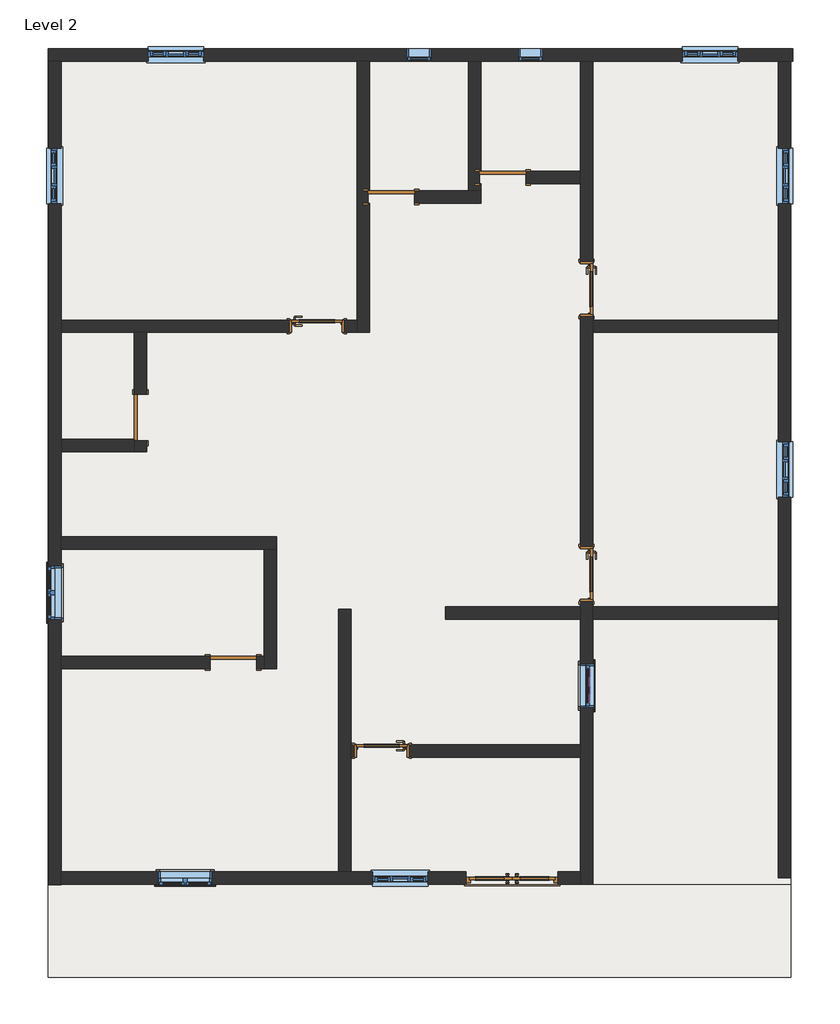
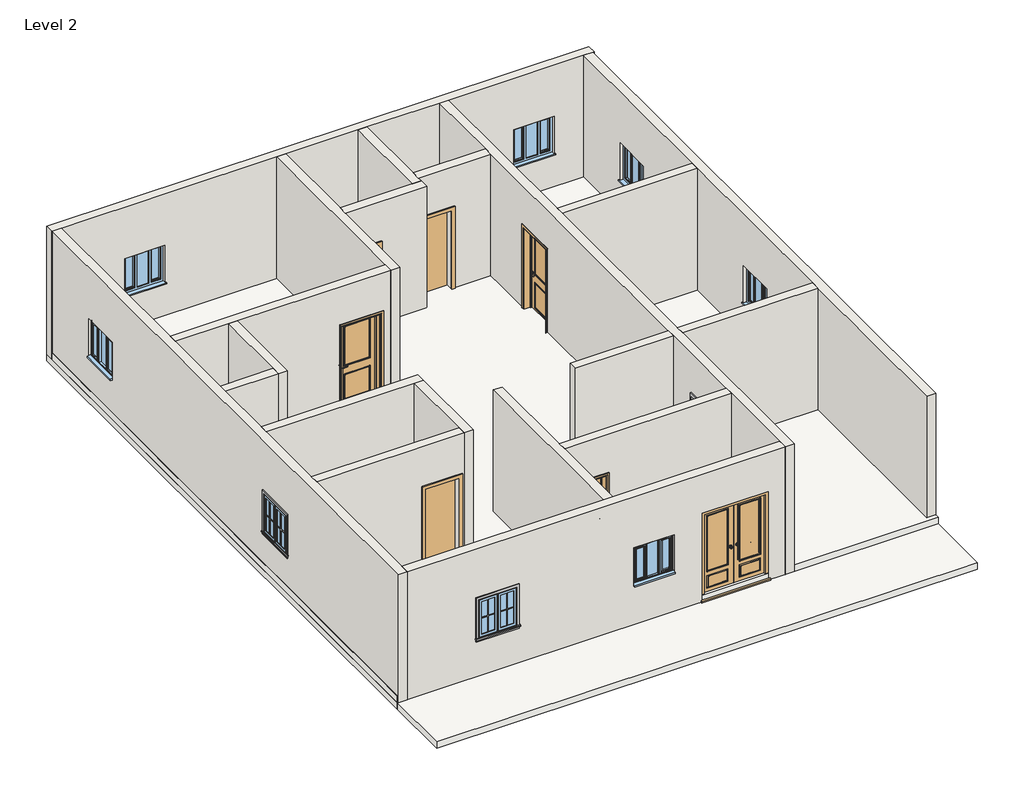
# One storey, incomplete: 19 walls, 12 proxies, 11 windows, 9 doors, 2 slabs, 1 roof.
# Revit data of these elements (continued)
# Element 40 (IfcWall, "9\"") (continued)
#   wall height = 10' - 0"
#   Phase Created = New Construction
#   Base Constraint = Level 2
#   Top Constraint = Level 3
#   Materials on its faces: "Default Wall"
# Elements 41, 42, 43 (IfcWall, "9\" wall")
#   Top Offset = 0' - 0"
#   Base Offset = 0' - 0"
#   wall height = 10' - 0"
#   Phase Created = New Construction
#   Base Constraint = Level 2
#   Top Constraint = Level 3
#   Materials on its faces: "Default Wall"
# Element 44 (IfcWindow, "Fixed : 16\" x 24\"")
#   Mark = "20"
#   Phase Created = New Construction
#   Materials on its faces: "Sash", "Glass"
# Element 45 (IfcWindow, "Fixed : 16\" x 24\"")
#   Mark = "21"
#   Phase Created = New Construction
#   Materials on its faces: "Sash", "Glass"
# Element 46 (IfcWindow, "Window-Casement-Double : 34\" x 36\"")
#   Mark = "12"
#   Window Inset = 0' - 0"
#   Interior Wall Closure = 0' - 2 1/4"
#   Frame Extension = 0' - 0 1/4"
#   Exterior Wall Closure = 0' - 1 1/4"
#   Interior Trim Visibility = yes
#   Exterior Trim Visibility = yes
#   Phase Created = New Construction
#   Materials on its faces: "Wood - Stained", "Glass", "Clad - White"
# Element 47 (IfcWindow, "Window-Casement-Double : 34\" x 36\"")
#   Mark = "13"
#   Window Inset = 0' - 0"
#   Interior Wall Closure = 0' - 2 1/4"
#   Frame Extension = 0' - 0 1/4"
#   Exterior Wall Closure = 0' - 1 1/4"
#   Interior Trim Visibility = yes
#   Exterior Trim Visibility = yes
#   Phase Created = New Construction
#   Materials on its faces: "Wood - Stained", "Glass", "Clad - White"
# Element 48 (IfcWindow, "Window-Double-Hung : 28\" x 46\"")
#   Mark = "22"
#   Window Inset = 0' - 0"
#   Interior Wall Closure = 0' - 1 1/2"
#   Frame Extension = 0' - 1 1/4"
#   Exterior Wall Closure = 0' - 0 1/2"
#   Interior Trim Visibility = yes
#   Indicator Visibility = yes
#   Exterior Trim Visibility = yes
#   Phase Created = New Construction
#   Materials on its faces: "Wood - Stained", "Glass", "Clad - White"
# Element 49 (IfcWindow, "Windows_Tpl_Plain : 910x910mm")
#   Mark = "14"
#   Phase Created = New Construction
#   Materials on its faces: "Window Frame", "Glass"
# Element 50 (IfcWindow, "Windows_Tpl_Plain : 910x910mm")
#   Mark = "17"
#   Phase Created = New Construction
#   Materials on its faces: "Window Frame", "Glass"
# Element 51 (IfcWindow, "Windows_Tpl_Plain : 910x910mm")
#   Mark = "18"
#   Phase Created = New Construction
#   Materials on its faces: "Window Frame", "Glass"
# Element 52 (IfcWindow, "Windows_Tpl_Plain : 910x910mm")
#   Mark = "19"
#   Phase Created = New Construction
#   Materials on its faces: "Window Frame", "Glass"
# Element 53 (IfcWindow, "Windows_Tpl_Plain : 910x910mm")
#   Mark = "15"
#   Phase Created = New Construction
#   Materials on its faces: "Window Frame", "Glass"
# Element 54 (IfcWindow, "Windows_Tpl_Plain : 910x910mm")
#   Mark = "16"
#   Phase Created = New Construction
#   Materials on its faces: "Window Frame", "Glass"
# Materials
#   "Door - Panel": class "Wood", colour RGB 210 159 95, transparency 0, Cost = 0
#   "Door - Glazing": colour RGB 0 0 255, transparency 0.75
#   "Door - Frame/Mullion": class "Wood", colour RGB 212 179 113, transparency 0
#   "Door - Handle": colour RGB 247 247 247, transparency 0
#   "Door - Architrave": class "Wood", colour RGB 154 90 5, transparency 0
#   "Door - Frame": colour RGB 118 70 51, transparency 0, Cost = 0
#   "Glass": class "Glass", colour RGB 0 128 192, transparency 0.75, Description = "Soda Lime Glass", Cost = 0
#   "Sash": class "Wood", colour RGB 224 178 126, transparency 0, Cost = 0
#   "Wood - Stained": class "Wood", colour RGB 224 178 126, transparency 0, Cost = 0
#   "Clad - White": class "Wood", colour RGB 242 242 238, transparency 0, Cost = 0
#   "Window Frame": colour RGB 249 249 249, transparency 0
#   "Default Roof": colour RGB 88 101 114, transparency 0, Cost = 0
#   "Default Floor": colour RGB 128 128 128, transparency 0, Cost = 0
#   "Default Wall": colour RGB 128 128 128, transparency 0, Cost = 0
